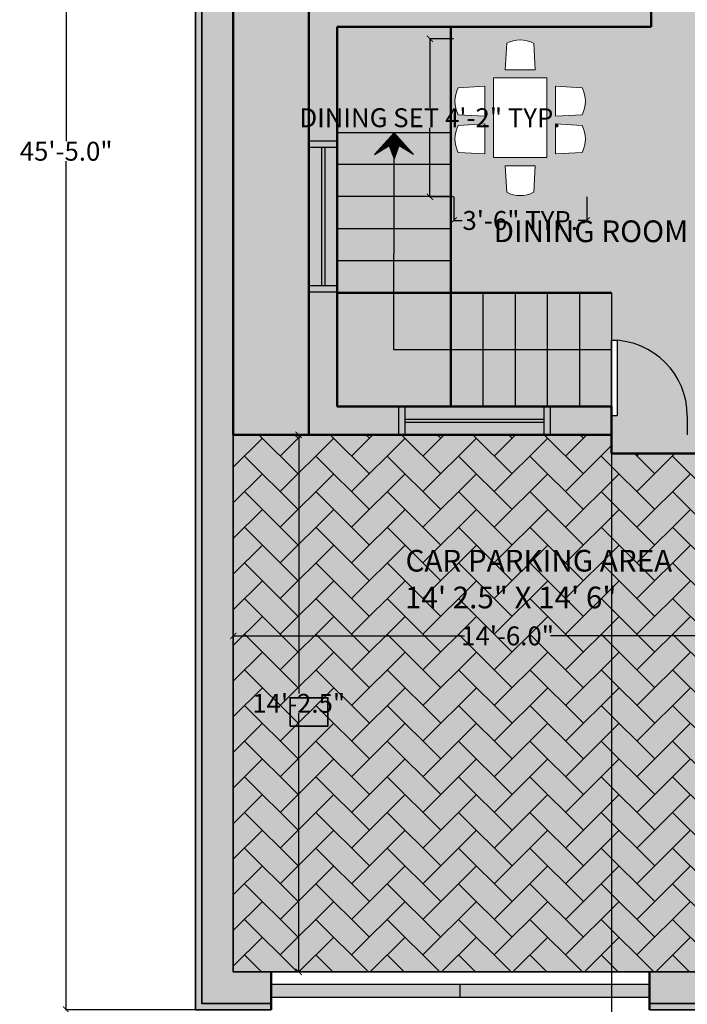
# Model space of a CAD drawing. Units: inches. Extents: x 528 to 2620, y -1066 to 798.
# Tile 2 of 41: x 528 to 740, y 211 to 523. Entities that reach past the tile are written whole.
import ezdxf

# ---------------------------------------------------------------- set-up
doc = ezdxf.new("R2010")
doc.units = ezdxf.units.IN
doc.header["$MEASUREMENT"] = 0
for name, color, linetype, lineweight in [('A-ANNO-DIMS', 2, 'Continuous', 18), ('A-AREA-IDEN', 7, 'Continuous', 18), ('A-COLS', 1, 'Continuous', 35), ('A-Door', 2, 'Continuous', 25), ('A-FLOR-PATT', 9, 'Continuous', 13), ('A-FLOR-STRS', 6, 'Continuous', 25), ('A-FURN', 30, 'Continuous', 18), ('A-GLAZ', 3, 'Continuous', 25), ('A-WALL', 7, 'Continuous', 50), ('A-WALL-PATT', 8, 'Continuous', 13), ('C-PROP', 5, 'Continuous', 35)]:
    doc.layers.add(name, color=color, linetype=linetype, lineweight=lineweight)
doc.styles.get("Standard").update_dxf_attribs({"font": 'arial.ttf'})
doc.dimstyles.get("Standard").update_dxf_attribs({"dimtxt": 6, "dimasz": 2, "dimexe": 0.18, "dimexo": 0.0625, "dimgap": 0.09, "dimtad": 0, "dimtih": 1, "dimtoh": 1, "dimdec": 1, "dimzin": 0, "dimdsep": 46, "dimlunit": 3, "dimtxsty": 'Standard', "dimblk": 'ARCHTICK', "dimcen": 0.09, "dimadec": 0, "dimazin": 0, "dimtfac": 1, "dimtdec": 1, "dimtofl": 0, "dimtmove": 0, "dimatfit": 3, "dimfxl": 1, "dimtolj": 1, "dimtzin": 0, "dimarcsym": 0})

# ---------------------------------------------------------------- blocks, each defined once
blk = doc.blocks.new('*U3')
for p, q in [((0, 0), (0, -6)), ((24, 0), (24, -6))]:
    blk.add_line(p, q)
blk.add_lwpolyline([(0, 0), (0, 24), (1.75, 24), (1.75, 0)], close=True)
blk.add_arc((0, 0), 24, 0, 90)
blk = doc.blocks.new('table-11')
at = {"color": 0, "linetype": 'ByBlock'}
for p, q in [((-1.122, 0.533), (-1.144, 0.134)), ((-0.716, 0.533), (-0.694, 0.134)), ((-0.554, 0.533), (-0.576, 0.134)), ((-0.148, 0.533), (-0.126, 0.134)), ((0, 0), (-1.2, 0)), ((-1.2, -0.8), (-1.2, 0)), ((-1.144, 0.134), (-0.694, 0.134)), ((-0.576, 0.134), (-0.126, 0.134)), ((0, -0.8), (0, 0)), ((-1.723, -0.197), (-1.324, -0.175)), ((-1.324, -0.625), (-1.324, -0.175)), ((0.523, -0.197), (0.124, -0.175)), ((0.124, -0.625), (0.124, -0.175)), ((-1.723, -0.603), (-1.324, -0.625)), ((0.523, -0.603), (0.124, -0.625)), ((0, -0.8), (-1.2, -0.8)), ((-1.144, -0.934), (-0.694, -0.934)), ((-1.122, -1.333), (-1.144, -0.934)), ((-0.716, -1.333), (-0.694, -0.934)), ((-0.576, -0.934), (-0.126, -0.934)), ((-0.554, -1.333), (-0.576, -0.934)), ((-0.148, -1.333), (-0.126, -0.934))]:
    blk.add_line(p, q, dxfattribs=at)
for centre, start, end in [((-0.919, 0.159), 61.4891, 118.5109), ((-0.351, 0.159), 61.4891, 118.5109), ((-1.349, -0.4), 151.4891, 208.5109), ((0.149, -0.4), 331.4891, 28.5109), ((-0.919, -0.959), 241.4891, 298.5109), ((-0.351, -0.959), 241.4891, 298.5109)]:
    blk.add_arc(centre, 0.425, start, end, dxfattribs=at)
blk = doc.blocks.new('_ArchTick')
at = {"color": 0, "linetype": 'ByBlock', "const_width": 0.15}
blk.add_lwpolyline([(-0.5, -0.5), (0.5, 0.5)], dxfattribs=at)
blk = doc.blocks.new('*D12')
at = {"layer": 'A-ANNO-DIMS', "color": 0, "lineweight": -2, "transparency": 16777216}
for p, q in [((584, 753.92), (542.88, 753.92)), ((543.06, 753.92), (543.06, 484.58)), ((543.06, 208.92), (543.06, 478.27)), ((584, 208.92), (542.88, 208.92))]:
    blk.add_line(p, q, dxfattribs=at)
at = {"layer": 'Defpoints', "color": 0, "transparency": 16777216}
for p in [(584.06, 753.92), (543.06, 208.92), (584.06, 208.92)]:
    blk.add_point(p, dxfattribs=at)
at = {"layer": 'A-ANNO-DIMS', "color": 0, "lineweight": -2, "transparency": 16777216, "xscale": 2, "yscale": 2, "zscale": 2}
for p, rotation in [((543.06, 753.92), 90), ((543.06, 208.92), 270)]:
    blk.add_blockref('_ArchTick', p, dxfattribs=dict(at, rotation=rotation))
at = {"layer": 'A-ANNO-DIMS', "color": 0, "transparency": 16777216, "insert": (543.06, 481.42), "char_height": 6, "attachment_point": 5}
blk.add_mtext('\\A1;45\'-5.0"', dxfattribs=at)
blk = doc.blocks.new('*D37')
at = {"layer": 'A-ANNO-DIMS', "color": 0, "lineweight": -2, "transparency": 16777216}
for p, q in [((596.06, 330.11), (596.06, 327.39)), ((770.06, 330.11), (770.06, 327.39)), ((596.06, 327.57), (669.45, 327.57)), ((770.06, 327.57), (696.67, 327.57))]:
    blk.add_line(p, q, dxfattribs=at)
at = {"layer": 'Defpoints', "color": 0, "transparency": 16777216}
for p in [(596.06, 330.17), (770.06, 330.17), (596.06, 327.57)]:
    blk.add_point(p, dxfattribs=at)
at = {"layer": 'A-ANNO-DIMS', "color": 0, "lineweight": -2, "transparency": 16777216, "xscale": 2, "yscale": 2, "zscale": 2, "rotation": 180}
blk.add_blockref('_ArchTick', (596.06, 327.57), dxfattribs=at)
at = {"layer": 'A-ANNO-DIMS', "color": 0, "lineweight": -2, "transparency": 16777216, "xscale": 2, "yscale": 2, "zscale": 2}
blk.add_blockref('_ArchTick', (770.06, 327.57), dxfattribs=at)
at = {"layer": 'A-ANNO-DIMS', "color": 0, "transparency": 16777216, "insert": (683.06, 327.57), "char_height": 6, "attachment_point": 5}
blk.add_mtext('\\A1;14\'-6.0"', dxfattribs=at)
blk = doc.blocks.new('*D38')
at = {"layer": 'A-ANNO-DIMS', "color": 0, "lineweight": -2, "transparency": 16777216}
for p, q in [((602.94, 391.42), (617, 391.42)), ((616.82, 391.42), (616.82, 309.33)), ((616.82, 220.92), (616.82, 303.02)), ((602.94, 220.92), (617, 220.92))]:
    blk.add_line(p, q, dxfattribs=at)
at = {"layer": 'Defpoints', "color": 0, "transparency": 16777216}
for p in [(602.87, 391.42), (602.87, 220.92), (616.82, 220.92)]:
    blk.add_point(p, dxfattribs=at)
at = {"layer": 'A-ANNO-DIMS', "color": 0, "lineweight": -2, "transparency": 16777216, "xscale": 2, "yscale": 2, "zscale": 2}
for p, rotation in [((616.82, 391.42), 90), ((616.82, 220.92), 270)]:
    blk.add_blockref('_ArchTick', p, dxfattribs=dict(at, rotation=rotation))
at = {"layer": 'A-ANNO-DIMS', "color": 0, "transparency": 16777216, "insert": (616.82, 306.17), "char_height": 6, "attachment_point": 5}
blk.add_mtext('\\A1;14\'-2.5"', dxfattribs=at)
blk = doc.blocks.new('WIN-1200')
for p, q in [((677.56, 718.92), (725.56, 718.92)), ((677.56, 709.92), (677.56, 718.92)), ((679.56, 709.92), (679.56, 718.92)), ((723.56, 718.92), (723.56, 709.92)), ((725.56, 718.92), (725.56, 709.92)), ((679.56, 714.92), (723.56, 714.92)), ((679.56, 713.92), (723.56, 713.92)), ((725.56, 709.92), (677.56, 709.92))]:
    blk.add_line(p, q)
blk = doc.blocks.new('*D48')
at = {"layer": 'A-ANNO-DIMS', "color": 0, "lineweight": -2, "transparency": 16777216}
for p, q in [((665.92, 517.14), (658.27, 517.14)), ((658.45, 517.14), (658.45, 495.24)), ((658.45, 466.96), (658.45, 488.86)), ((665.92, 466.96), (658.27, 466.96))]:
    blk.add_line(p, q, dxfattribs=at)
at = {"layer": 'Defpoints', "color": 0, "transparency": 16777216}
for p in [(658.45, 517.14), (665.98, 517.14), (665.98, 466.96)]:
    blk.add_point(p, dxfattribs=at)
at = {"layer": 'A-ANNO-DIMS', "color": 0, "lineweight": -2, "transparency": 16777216, "xscale": 2, "yscale": 2, "zscale": 2}
for p, rotation in [((658.45, 517.14), 90), ((658.45, 466.96), 270)]:
    blk.add_blockref('_ArchTick', p, dxfattribs=dict(at, rotation=rotation))
at = {"layer": 'A-ANNO-DIMS', "color": 0, "transparency": 16777216, "insert": (658.45, 492.05), "char_height": 6, "attachment_point": 5}
blk.add_mtext('\\A1;DINING SET 4\'-2" TYP.', dxfattribs=at)
blk = doc.blocks.new('*D49')
at = {"layer": 'A-ANNO-DIMS', "color": 0, "lineweight": -2, "transparency": 16777216}
for p, q in [((665.98, 466.9), (665.98, 459.26)), ((708.15, 466.9), (708.15, 459.26)), ((665.98, 459.44), (668.69, 459.44)), ((708.15, 459.44), (705.44, 459.44))]:
    blk.add_line(p, q, dxfattribs=at)
at = {"layer": 'Defpoints', "color": 0, "transparency": 16777216}
for p in [(665.98, 466.96), (708.15, 466.96), (665.98, 459.44)]:
    blk.add_point(p, dxfattribs=at)
at = {"layer": 'A-ANNO-DIMS', "color": 0, "lineweight": -2, "transparency": 16777216, "xscale": 2, "yscale": 2, "zscale": 2, "rotation": 180}
blk.add_blockref('_ArchTick', (665.98, 459.44), dxfattribs=at)
at = {"layer": 'A-ANNO-DIMS', "color": 0, "lineweight": -2, "transparency": 16777216, "xscale": 2, "yscale": 2, "zscale": 2}
blk.add_blockref('_ArchTick', (708.15, 459.44), dxfattribs=at)
at = {"layer": 'A-ANNO-DIMS', "color": 0, "transparency": 16777216, "insert": (687.06, 459.44), "char_height": 6, "attachment_point": 5}
blk.add_mtext('\\A1;3\'-6" TYP.', dxfattribs=at)
blk = doc.blocks.new('*D57')
at = {"layer": 'A-ANNO-DIMS', "color": 0, "lineweight": -2, "transparency": 16777216}
for p, q in [((716.06, 391.36), (716.06, 174.74)), ((764.06, 391.36), (764.06, 174.74)), ((716.06, 174.92), (731.87, 174.92)), ((764.06, 174.92), (748.24, 174.92))]:
    blk.add_line(p, q, dxfattribs=at)
at = {"layer": 'Defpoints', "color": 0, "transparency": 16777216}
for p in [(716.06, 391.42), (764.06, 391.42), (764.06, 174.92)]:
    blk.add_point(p, dxfattribs=at)
at = {"layer": 'A-ANNO-DIMS', "color": 0, "lineweight": -2, "transparency": 16777216, "xscale": 2, "yscale": 2, "zscale": 2, "rotation": 180}
blk.add_blockref('_ArchTick', (716.06, 174.92), dxfattribs=at)
at = {"layer": 'A-ANNO-DIMS', "color": 0, "lineweight": -2, "transparency": 16777216, "xscale": 2, "yscale": 2, "zscale": 2}
blk.add_blockref('_ArchTick', (764.06, 174.92), dxfattribs=at)
at = {"layer": 'A-ANNO-DIMS', "color": 0, "transparency": 16777216, "insert": (740.06, 174.92), "char_height": 6, "attachment_point": 5}
blk.add_mtext('\\A1;4\'-0"', dxfattribs=at)

msp = doc.modelspace()

# ---------------------------------------------------------------- hatches: boundary and pattern name
at = {"layer": 'A-COLS', "transparency": 33554687}
h = msp.add_hatch(color=256, dxfattribs=at)
h.dxf.hatch_style = 1
h.paths.add_polyline_path([(614.06, 307.96), (614.06, 298.96), (626.06, 298.96), (626.06, 307.96)])
at = {"layer": 'A-FLOR-PATT', "transparency": 33554607}
h = msp.add_hatch(dxfattribs=at)
h.set_pattern_fill('AR-HBONE', color=256, scale=2)
h.paths.add_polyline_path([(770.06, 391.42), (764.06, 391.42), (764.06, 385.42), (716.06, 385.42), (716.06, 391.42), (620.06, 391.42), (596.06, 391.42), (596.06, 220.92), (770.06, 220.92), (770.06, 268.92)])
at = {"layer": 'A-WALL-PATT', "transparency": 33554687}
h = msp.add_hatch(color=256, dxfattribs=at)
h.dxf.hatch_style = 1
h.paths.add_polyline_path([(944.06, 753.92), (584.06, 753.92), (584.06, 208.92), (608.06, 208.92), (608.06, 210.92), (586.06, 210.92), (586.06, 751.92), (942.06, 751.92), (942.06, 210.92), (728.06, 210.92), (728.06, 208.92), (944.06, 208.92)])
h = msp.add_hatch(color=256, dxfattribs=at)
h.dxf.hatch_style = 1
h.paths.add_polyline_path([(942.06, 751.92), (586.06, 751.92), (586.06, 210.92), (608.06, 210.92), (608.06, 220.92), (596.06, 220.92), (596.06, 741.92), (932.06, 741.92), (932.06, 220.92), (770.06, 220.92), (728.06, 220.92), (728.06, 210.92), (942.06, 210.92)])
at = {"layer": 'A-WALL-PATT', "transparency": 33554475}
h = msp.add_hatch(color=256, dxfattribs=at)
h.dxf.hatch_style = 1
h.paths.add_polyline_path([(620.06, 718.92), (908.06, 718.92), (908.06, 268.92), (770.06, 268.92), (770.06, 220.92), (932.06, 220.92), (932.06, 741.92), (596.06, 741.92), (596.06, 391.42), (620.06, 391.42)])
at = {"layer": 'A-WALL-PATT', "transparency": 33554687}
h = msp.add_hatch(color=256, dxfattribs=at)
h.dxf.hatch_style = 1
h.paths.add_polyline_path([(861.06, 273.92), (817.06, 273.92), (817.06, 272.92), (861.06, 272.92)])
h.paths.add_polyline_path([(817.06, 277.92), (815.06, 277.92), (815.06, 268.92), (817.06, 268.92)])
h.paths.add_polyline_path([(908.06, 397.92), (899.06, 397.92), (899.06, 395.92), (908.06, 395.92)])
h.paths.add_polyline_path([(908.06, 443.92), (899.06, 443.92), (899.06, 441.92), (908.06, 441.92)])
h.paths.add_polyline_path([(904.06, 441.92), (903.06, 441.92), (903.06, 397.92), (904.06, 397.92)])
h.paths.add_polyline_path([(625.06, 561.42), (624.06, 561.42), (624.06, 537.42), (625.06, 537.42)])
h.paths.add_polyline_path([(648.75, 334.44), (720.04, 334.44), (720.04, 345), (648.75, 345)], flags=9)
h.paths.add_polyline_path([(819.73, 323.15), (880.33, 323.15), (880.33, 333.71), (819.73, 333.71)], flags=9)
h.paths.add_polyline_path([(779.9, 680.61), (821.76, 680.61), (821.76, 691.17), (779.9, 691.17)], flags=9)
h.paths.add_polyline_path([(779.88, 692.36), (817.14, 692.36), (817.14, 703.06), (779.88, 703.06)], flags=9)
h.paths.add_polyline_path([(799.99, 453.88), (860.59, 453.88), (860.59, 464.44), (799.99, 464.44)], flags=9)
h.paths.add_polyline_path([(650.87, 539.4), (708.78, 539.4), (708.78, 549.95), (650.87, 549.95)], flags=9)
h.paths.add_polyline_path([(788.5, 612.01), (849.1, 612.01), (849.1, 622.56), (788.5, 622.56)], flags=9)
h.paths.add_polyline_path([(639.54, 648.31), (700.13, 648.31), (700.13, 658.87), (639.54, 658.87)], flags=9)
h.paths.add_polyline_path([(648.91, 346.09), (747.71, 346.09), (747.71, 356.78), (648.91, 356.78)], flags=9)
h.paths.add_polyline_path([(676.86, 450.66), (746.74, 450.66), (746.74, 461.36), (676.86, 461.36)], flags=9)
h.paths.add_polyline_path([(819.71, 334.95), (865.53, 334.95), (865.53, 345.64), (819.71, 345.64)], flags=9)
h.paths.add_polyline_path([(806.3, 467.75), (874.05, 467.75), (874.05, 478.44), (806.3, 478.44)], flags=9)
h.paths.add_polyline_path([(653.23, 552.28), (690.5, 552.28), (690.5, 562.98), (653.23, 562.98)], flags=9)
h.paths.add_polyline_path([(789.9, 623.41), (843.21, 623.41), (843.21, 634.1), (789.9, 634.1)], flags=9)
h.paths.add_polyline_path([(639.77, 662.1), (693.08, 662.1), (693.08, 672.8), (639.77, 672.8)], flags=9)
h.paths.add_polyline_path([(801.59, 242.91), (846.33, 242.91), (846.33, 253.6), (801.59, 253.6)], flags=9)
h.paths.add_polyline_path([(925.36, 593.98), (925.36, 674.06), (914.67, 674.06), (914.67, 593.98)], flags=9)
h.paths.add_polyline_path([(612.56, 593.98), (612.56, 674.06), (601.87, 674.06), (601.87, 593.98)], flags=9)
h.paths.add_polyline_path([(723.31, 726.56), (803.39, 726.56), (803.39, 737.25), (723.31, 737.25)], flags=9)
at = {"layer": 'A-WALL-PATT', "transparency": 33554521}
h = msp.add_hatch(color=256, dxfattribs=at)
h.dxf.hatch_style = 1
h.paths.add_polyline_path([(629.06, 709.92), (677.56, 709.92), (677.56, 718.92), (620.06, 718.92), (620.06, 667.92), (629.06, 667.92)])
h.paths.add_polyline_path([(790.56, 718.92), (725.56, 718.92), (725.56, 709.92), (774.06, 709.92), (774.06, 577.92), (768.48, 577.92), (768.56, 573.42), (774.06, 573.42), (774.06, 567.42), (778.56, 567.42), (778.56, 669.42), (831.06, 669.42), (831.06, 675.92), (826.56, 675.92), (826.56, 673.92), (778.56, 673.92), (778.56, 709.92), (790.56, 709.92)])
h.paths.add_polyline_path([(908.06, 718.92), (879.06, 718.92), (879.06, 709.92), (899.06, 709.92), (899.06, 641.67), (908.06, 641.67)])
h.paths.add_polyline_path([(629.06, 619.92), (620.06, 619.92), (620.06, 561.42), (629.06, 561.42), (629.06, 573.42), (724.06, 573.42), (724.06, 569.42), (728.56, 569.42), (728.56, 577.92), (629.06, 577.92)])
h.paths.add_polyline_path([(779.06, 391.42), (779.06, 400.42), (770.06, 400.42), (764.06, 400.42), (764.06, 397.42), (764.06, 391.42), (770.06, 391.42), (770.06, 268.92), (815.06, 268.92), (815.06, 277.92), (779.06, 277.92), (779.06, 359.77)])
h.paths.add_polyline_path([(908.06, 395.92), (899.06, 395.92), (851.06, 395.92), (851.06, 391.42), (899.06, 391.42), (899.06, 277.92), (863.06, 277.92), (863.06, 268.92), (908.06, 268.92)])
h.paths.add_polyline_path([(908.06, 593.67), (899.06, 593.67), (899.06, 525.42), (778.56, 525.42), (778.56, 527.17), (774.06, 527.17), (774.06, 520.92), (899.06, 520.92), (899.06, 443.92), (908.06, 443.92)])
h.paths.add_polyline_path([(629.06, 520.92), (728.56, 520.92), (728.56, 545.42), (724.06, 545.42), (724.06, 525.42), (629.06, 525.42), (629.06, 537.42), (620.06, 537.42), (620.06, 484.67), (629.06, 484.67)])
h.paths.add_polyline_path([(629.06, 436.67), (620.06, 436.67), (620.06, 391.42), (648.56, 391.42), (648.56, 400.42), (629.06, 400.42)])
h.paths.add_polyline_path([(716.06, 397.42), (716.06, 400.42), (696.56, 400.42), (696.56, 391.42), (716.06, 391.42)])
at = {"layer": 'A-WALL-PATT', "transparency": 33554681}
h = msp.add_hatch(color=256, dxfattribs=at)
h.dxf.hatch_style = 1
h.paths.add_polyline_path([(629.06, 665.92), (625.06, 665.92), (625.06, 621.92), (629.06, 621.92)])
h.paths.add_polyline_path([(624.06, 665.92), (620.06, 665.92), (620.06, 621.92), (624.06, 621.92)])
h.paths.add_polyline_path([(723.56, 713.92), (679.56, 713.92), (679.56, 709.92), (723.56, 709.92)])
h.paths.add_polyline_path([(723.56, 718.92), (679.56, 718.92), (679.56, 714.92), (723.56, 714.92)])
h.paths.add_polyline_path([(814.56, 713.92), (790.56, 713.92), (790.56, 709.92), (814.56, 709.92)])
h.paths.add_polyline_path([(814.56, 718.92), (790.56, 718.92), (790.56, 714.92), (814.56, 714.92)])
h.paths.add_polyline_path([(877.06, 713.92), (833.06, 713.92), (833.06, 709.92), (877.06, 709.92)])
h.paths.add_polyline_path([(877.06, 718.92), (833.06, 718.92), (833.06, 714.92), (877.06, 714.92)])
h.paths.add_polyline_path([(908.06, 639.67), (904.06, 639.67), (904.06, 595.67), (908.06, 595.67)])
h.paths.add_polyline_path([(903.06, 639.67), (899.06, 639.67), (899.06, 595.67), (903.06, 595.67)])
h.paths.add_polyline_path([(908.06, 441.92), (904.06, 441.92), (904.06, 397.92), (908.06, 397.92)])
h.paths.add_polyline_path([(903.06, 441.92), (899.06, 441.92), (899.06, 397.92), (903.06, 397.92)])
h.paths.add_polyline_path([(861.06, 272.92), (817.06, 272.92), (817.06, 268.92), (861.06, 268.92)])
h.paths.add_polyline_path([(861.06, 277.92), (817.06, 277.92), (817.06, 273.92), (861.06, 273.92)])
h.paths.add_polyline_path([(694.56, 395.42), (650.56, 395.42), (650.56, 391.42), (694.56, 391.42)])
h.paths.add_polyline_path([(694.56, 400.42), (650.56, 400.42), (650.56, 396.42), (694.56, 396.42)])
h.paths.add_polyline_path([(629.06, 482.67), (625.06, 482.67), (625.06, 438.67), (629.06, 438.67)])
h.paths.add_polyline_path([(624.06, 482.67), (620.06, 482.67), (620.06, 438.67), (624.06, 438.67)])
h.paths.add_polyline_path([(629.06, 561.42), (625.06, 561.42), (625.06, 537.42), (629.06, 537.42)])
h.paths.add_polyline_path([(624.06, 561.42), (620.06, 561.42), (620.06, 537.42), (624.06, 537.42)])
h = msp.add_hatch(color=256, dxfattribs=at)
h.dxf.hatch_style = 1
h.paths.add_polyline_path([(625.06, 665.92), (624.06, 665.92), (624.06, 621.92), (625.06, 621.92)])
h.paths.add_polyline_path([(629.06, 667.92), (620.06, 667.92), (620.06, 665.92), (629.06, 665.92)])
h.paths.add_polyline_path([(629.06, 621.92), (620.06, 621.92), (620.06, 619.92), (629.06, 619.92)])
h.paths.add_polyline_path([(723.56, 714.92), (679.56, 714.92), (679.56, 713.92), (723.56, 713.92)])
h.paths.add_polyline_path([(725.56, 718.92), (723.56, 718.92), (723.56, 709.92), (725.56, 709.92)])
h.paths.add_polyline_path([(679.56, 718.92), (677.56, 718.92), (677.56, 709.92), (679.56, 709.92)])
h.paths.add_polyline_path([(814.56, 714.92), (790.56, 714.92), (790.56, 713.92), (814.56, 713.92)])
h.paths.add_polyline_path([(877.06, 714.92), (833.06, 714.92), (833.06, 713.92), (877.06, 713.92)])
h.paths.add_polyline_path([(879.06, 718.92), (877.06, 718.92), (877.06, 709.92), (879.06, 709.92)])
h.paths.add_polyline_path([(833.06, 718.92), (831.06, 718.92), (831.06, 709.92), (833.06, 709.92)])
h.paths.add_polyline_path([(650.56, 400.42), (648.56, 400.42), (648.56, 391.42), (650.56, 391.42)])
h.paths.add_polyline_path([(694.56, 396.42), (650.56, 396.42), (650.56, 395.42), (694.56, 395.42)])
h.paths.add_polyline_path([(696.56, 400.42), (694.56, 400.42), (694.56, 391.42), (696.56, 391.42)])
h.paths.add_polyline_path([(629.06, 438.67), (620.06, 438.67), (620.06, 436.67), (629.06, 436.67)])
h.paths.add_polyline_path([(629.06, 484.67), (620.06, 484.67), (620.06, 482.67), (629.06, 482.67)])
h.paths.add_polyline_path([(625.06, 482.67), (624.06, 482.67), (624.06, 438.67), (625.06, 438.67)])
at = {"layer": 'A-WALL-PATT', "transparency": 33554590}
h = msp.add_hatch(color=256, dxfattribs=at)
h.dxf.hatch_style = 1
h.paths.add_polyline_path([(774.06, 709.92), (629.06, 709.92), (629.06, 577.92), (728.56, 577.92), (728.56, 579.42), (728.56, 619.42), (730.31, 619.42), (730.31, 619.38, -0.401453), (768.56, 579.42), (768.56, 577.92), (774.06, 577.92)])
h.paths.add_polyline_path([(723.9, 686.06), (723.97, 686.06), (723.83, 686.13)], flags=0)
h.paths.add_polyline_path([(722.79, 642.7), (722.89, 642.76), (722.89, 684.99), (722.65, 685.24), (722.65, 685.82), (723.08, 686.26), (723.53, 686.26), (723.97, 686.06), (724.74, 686.13), (770.7, 686.13), (770.78, 686.14), (771.13, 686.27), (771.69, 686.09), (771.94, 685.48), (771.67, 684.9), (771.58, 684.87), (771.58, 642.78), (771.88, 642.51), (771.88, 641.92), (771.51, 641.46), (770.85, 641.46), (770.4, 641.83), (770.4, 641.55), (724.74, 641.55), (723.99, 641.7), (723.44, 641.41), (722.88, 641.59), (722.6, 642.14)], flags=16)
h.paths.add_polyline_path([(723.99, 641.7), (723.99, 641.71), (723.99, 641.7)], flags=0)
h.paths.add_polyline_path([(722.89, 642.73), (722.89, 684.99), (722.65, 685.24), (722.65, 685.82), (723.08, 686.26), (723.29, 686.26), (722.99, 686.17), (722.79, 685.97), (722.65, 685.68), (722.65, 685.43), (722.75, 685.14), (722.94, 684.94), (723.24, 684.81), (723.48, 684.81), (723.78, 684.9), (723.98, 685.1), (724.17, 685.49), (724.12, 685.64), (724.12, 685.25), (723.63, 684.75), (723.63, 642.96), (724.12, 642.51), (724.12, 641.89), (723.66, 641.46), (723.08, 641.46), (722.65, 641.9), (722.65, 642.48)], flags=0)
h.paths.add_polyline_path([(722.65, 642.29), (722.65, 642.04), (722.79, 641.75), (723.08, 641.46), (723.29, 641.46), (722.88, 641.59), (722.6, 642.14)], flags=0)
h.paths.add_polyline_path([(770.75, 686.13), (770.58, 686.13), (770.55, 686.06)], flags=0)
h.paths.add_polyline_path([(743.3, 645.29), (753.23, 659.4), (748.69, 663.75), (753.23, 668.54), (743.3, 682.46), (743.79, 682.59), (744.14, 682.68), (744.53, 682.93), (744.63, 683.08), (745.02, 683.33), (744.53, 684.07), (744.78, 684.16), (744.87, 684.31), (745.51, 684.4), (746.08, 684.65), (746.47, 684.65), (746.82, 684.81), (747.46, 685.03), (747.71, 685.14), (748.2, 685.28), (748.39, 685.52), (748.86, 685.52), (749.99, 686.13), (753.49, 676.03), (757.38, 680.15), (757.79, 679.76), (758.04, 680.65), (758.29, 681.23), (758.29, 682.05), (758.02, 682.59), (757.87, 683.17), (757.82, 683.78), (758.39, 684.07), (758.98, 684.2), (759.62, 684.16), (760.21, 683.96), (760.75, 683.67), (761.86, 683.67), (762.4, 683.96), (762.99, 684.11), (763.63, 684.11), (764.2, 683.96), (764.74, 683.67), (766.12, 683.67), (766.66, 683.96), (767.25, 684.16), (767.87, 684.2), (768.46, 684.07), (769.05, 683.78), (769, 683.17), (768.85, 682.59), (768.55, 682.05), (768.55, 681.23), (768.8, 680.65), (769.09, 679.75), (768.95, 678.83), (768.8, 678.23), (768.55, 677.65), (768.55, 676.82), (768.8, 676.24), (769.09, 675.34), (768.95, 674.42), (768.8, 673.82), (768.55, 673.28), (768.55, 672.41), (768.8, 671.87), (769, 671.29), (769.05, 670.64), (768.95, 670.02), (768.8, 669.41), (768.55, 668.87), (768.55, 668), (768.97, 667.24), (769.05, 666.28), (769.05, 665.56), (768.46, 665.32), (767.87, 665.16), (767.25, 665.16), (766.66, 665.36), (766.12, 665.7), (764.74, 665.7), (763.94, 665.2), (762.99, 665.2), (762.4, 665.36), (761.86, 665.7), (761, 665.7), (762.7, 664.09), (760.74, 662.03), (761.86, 662.03), (762.4, 662.32), (763.34, 662.55), (764.25, 662.32), (764.79, 662.03), (766.12, 662.03), (766.66, 662.32), (767.25, 662.52), (767.87, 662.56), (768.51, 662.43), (769.05, 662.12), (769.05, 661.4), (769.05, 660.8), (768.85, 660.21), (768.55, 659.68), (768.55, 658.85), (768.85, 658.27), (769, 657.66), (769.07, 656.75), (768.85, 655.85), (768.55, 655.27), (768.55, 654.44), (768.85, 653.86), (769.07, 652.96), (769, 652.05), (768.85, 651.44), (768.55, 650.91), (768.55, 650.03), (768.85, 649.5), (769, 648.91), (769.05, 648.26), (769, 647.64), (768.85, 647.03), (768.55, 646.5), (768.55, 645.62), (768.85, 645.09), (769.05, 644.55), (769.05, 643.9), (768.51, 643.65), (767.87, 643.52), (767.25, 643.52), (766.66, 643.72), (766.12, 644.06), (764.79, 644.06), (764.25, 643.72), (763.34, 643.49), (762.4, 643.72), (761.86, 644.06), (760.8, 644.06), (760.26, 643.72), (759.67, 643.52), (759.03, 643.52), (758.39, 643.65), (757.87, 643.9), (757.87, 644.55), (758.04, 645.09), (758.34, 645.62), (758.34, 646.5), (758.04, 647.03), (757.92, 647.64), (757.87, 648.06), (757.38, 647.59), (753.42, 651.77), (749.99, 641.62), (749.5, 641.71), (749.35, 641.95), (748.54, 642.45), (747.31, 642.94), (746.65, 642.94), (746.33, 643.18), (745.51, 643.57), (744.53, 643.65), (745.01, 644.4), (744.63, 644.64), (744.14, 644.89), (743.79, 645.13)], flags=0)
h.paths.add_polyline_path([(755.66, 654.93), (756.54, 654.69), (757.53, 654.33), (756.64, 654.58)], flags=0)
h.paths.add_polyline_path([(758.34, 649.2), (758.34, 648.71), (758.59, 644.3), (758.59, 648.8)], flags=0)
h.paths.add_polyline_path([(758.34, 649.29), (758.09, 649.7), (758.36, 649.17)], flags=0)
h.paths.add_polyline_path([(755.66, 672.79), (756.49, 673.04), (757.36, 673.35), (757.35, 673.36), (756.64, 673.15)], flags=0)
h.paths.add_polyline_path([(760.26, 639.64), (771.41, 639.64), (771.41, 624.04), (760.26, 624.04)], flags=16)
h.paths.add_polyline_path([(761.38, 638.53), (770.29, 638.53), (770.29, 625.15), (761.38, 625.15)], flags=0)
edge = h.paths.add_edge_path(flags=0)
edge.add_ellipse((765.84, 631.84), major_axis=(-2.24, 2.24), ratio=1, start_angle=-45, end_angle=45, ccw=False)
edge.add_ellipse((765.84, 631.84), major_axis=(-2.24, 2.24), ratio=1, start_angle=-135, end_angle=-45, ccw=False)
edge.add_ellipse((765.84, 631.84), major_axis=(-2.24, 2.24), ratio=1, start_angle=135, end_angle=-135, ccw=False)
edge.add_ellipse((765.84, 631.84), major_axis=(-2.24, 2.24), ratio=1, start_angle=45, end_angle=135, ccw=False)
h.paths.add_polyline_path([(758.59, 683.42), (758.59, 678.92), (758.37, 678.58), (758.34, 678.43), (758.09, 678.05), (758.34, 678.52), (758.34, 679.01)], flags=0)
h.paths.add_polyline_path([(760.26, 688.04), (760.26, 703.64), (771.41, 703.64), (771.41, 688.04)], flags=16)
h.paths.add_polyline_path([(770.4, 685.39), (770.4, 685.85), (770.85, 686.22), (771.51, 686.22), (771.88, 685.76), (771.88, 685.17), (771.58, 684.9), (771.58, 642.78), (771.88, 642.51), (771.88, 641.92), (771.51, 641.46), (770.85, 641.46), (770.4, 641.83), (770.4, 642.29)], flags=0)
h.paths.add_polyline_path([(770.53, 642.68), (771.05, 643.01), (771.67, 642.77), (771.94, 642.2), (771.69, 641.59), (771.13, 641.41), (770.55, 641.62), (770.35, 642.13)], flags=16)
h.paths.add_polyline_path([(761.38, 689.15), (761.38, 702.53), (770.29, 702.53), (770.29, 689.15)], flags=0)
edge = h.paths.add_edge_path(flags=0)
edge.add_ellipse((765.84, 695.84), major_axis=(2.24, 2.24), ratio=1, start_angle=405, end_angle=495, ccw=False)
edge.add_ellipse((765.84, 695.84), major_axis=(2.24, 2.24), ratio=1, start_angle=675, end_angle=765, ccw=False)
edge.add_ellipse((765.84, 695.84), major_axis=(2.24, 2.24), ratio=1, start_angle=585, end_angle=675, ccw=False)
edge.add_ellipse((765.84, 695.84), major_axis=(2.24, 2.24), ratio=1, start_angle=495, end_angle=585, ccw=False)
h.paths.add_polyline_path([(770.7, 684.9), (770.94, 684.74), (771.41, 684.74), (771.73, 685.03), (771.88, 685.34), (771.88, 685.64), (771.69, 686.09), (771.58, 686.13), (771.88, 685.76), (771.88, 685.17), (771.41, 684.74), (770.85, 684.74)], flags=0)
h.paths.add_polyline_path([(899.06, 709.92), (831.06, 709.92), (831.06, 699.92), (829.81, 699.92), (829.81, 675.92), (831.06, 675.92), (831.06, 669.42), (778.56, 669.42), (778.56, 567.17), (780.06, 567.17), (820.06, 567.17), (820.06, 565.42), (820.02, 565.42, -0.401453), (780.06, 527.17), (778.56, 527.17), (778.56, 525.42), (899.06, 525.42)])
h.paths.add_polyline_path([(849.2, 636.01), (849.27, 636.02), (849.13, 636.08)], flags=0)
h.paths.add_polyline_path([(848.19, 634.95), (847.95, 635.2), (847.95, 635.78), (848.38, 636.22), (848.83, 636.22), (849.27, 636.02), (850.04, 636.08), (896, 636.08), (896.08, 636.1), (896.43, 636.22), (896.99, 636.05), (897.24, 635.43), (896.97, 634.86), (896.88, 634.83), (896.88, 592.74), (897.18, 592.47), (897.18, 591.88), (896.81, 591.42), (896.15, 591.42), (895.7, 591.79), (895.7, 591.51), (850.04, 591.51), (849.29, 591.66), (848.74, 591.37), (848.18, 591.54), (847.9, 592.1), (848.09, 592.65), (848.19, 592.71)], flags=16)
h.paths.add_polyline_path([(849.29, 591.66), (849.29, 591.66), (849.29, 591.66)], flags=16)
h.paths.add_polyline_path([(848.19, 634.95), (847.95, 635.2), (847.95, 635.78), (848.38, 636.22), (848.59, 636.22), (848.29, 636.13), (848.09, 635.93), (847.95, 635.64), (847.95, 635.39), (848.05, 635.1), (848.24, 634.9), (848.54, 634.76), (848.78, 634.76), (849.08, 634.85), (849.28, 635.05), (849.47, 635.44), (849.42, 635.59), (849.42, 635.21), (848.93, 634.7), (848.93, 592.92), (849.42, 592.47), (849.42, 591.84), (848.96, 591.42), (848.38, 591.42), (847.95, 591.86), (847.95, 592.44), (848.19, 592.69)], flags=0)
h.paths.add_polyline_path([(847.95, 592.25), (847.95, 592), (848.09, 591.71), (848.38, 591.42), (848.59, 591.42), (848.18, 591.54), (847.9, 592.1)], flags=16)
h.paths.add_polyline_path([(896.05, 636.08), (895.88, 636.08), (895.85, 636.01)], flags=0)
h.paths.add_polyline_path([(868.6, 632.41), (869.09, 632.55), (869.44, 632.64), (869.83, 632.88), (869.93, 633.04), (870.32, 633.28), (869.83, 634.02), (870.08, 634.11), (870.17, 634.27), (870.81, 634.36), (871.38, 634.61), (871.77, 634.61), (872.12, 634.76), (872.76, 634.99), (873.01, 635.1), (873.5, 635.23), (873.69, 635.48), (874.16, 635.48), (875.29, 636.08), (878.79, 625.99), (882.68, 630.11), (883.09, 629.71), (883.34, 630.6), (883.59, 631.18), (883.59, 632.01), (883.32, 632.55), (883.17, 633.13), (883.12, 633.73), (883.69, 634.02), (884.28, 634.16), (884.92, 634.11), (885.51, 633.91), (886.05, 633.62), (887.16, 633.62), (887.7, 633.91), (888.29, 634.07), (888.93, 634.07), (889.5, 633.91), (890.04, 633.62), (891.42, 633.62), (891.96, 633.91), (892.55, 634.11), (893.17, 634.16), (893.76, 634.02), (894.35, 633.73), (894.3, 633.13), (894.15, 632.55), (893.85, 632.01), (893.85, 631.18), (894.1, 630.6), (894.39, 629.71), (894.25, 628.79), (894.1, 628.18), (893.85, 627.6), (893.85, 626.77), (894.1, 626.19), (894.39, 625.3), (894.25, 624.38), (894.1, 623.78), (893.85, 623.24), (893.85, 622.37), (894.1, 621.83), (894.3, 621.25), (894.35, 620.6), (894.25, 619.97), (894.1, 619.37), (893.85, 618.83), (893.85, 617.96), (894.27, 617.2), (894.35, 616.23), (894.35, 615.52), (893.76, 615.27), (893.17, 615.12), (892.55, 615.12), (891.96, 615.32), (891.42, 615.65), (890.04, 615.65), (889.25, 615.16), (888.29, 615.16), (887.7, 615.32), (887.16, 615.65), (886.31, 615.65), (888, 614.04), (886.04, 611.98), (887.16, 611.98), (887.7, 612.27), (888.64, 612.5), (889.55, 612.27), (890.09, 611.98), (891.42, 611.98), (891.96, 612.27), (892.55, 612.48), (893.17, 612.52), (893.81, 612.39), (894.35, 612.07), (894.35, 611.36), (894.35, 610.75), (894.15, 610.17), (893.85, 609.63), (893.85, 608.81), (894.15, 608.22), (894.3, 607.62), (894.37, 606.7), (894.15, 605.81), (893.85, 605.22), (893.85, 604.4), (894.15, 603.81), (894.37, 602.92), (894.3, 602), (894.15, 601.4), (893.85, 600.86), (893.85, 599.99), (894.15, 599.45), (894.3, 598.87), (894.35, 598.22), (894.3, 597.59), (894.15, 596.99), (893.85, 596.45), (893.85, 595.58), (894.15, 595.04), (894.35, 594.51), (894.35, 593.86), (893.81, 593.61), (893.17, 593.48), (892.55, 593.48), (891.96, 593.68), (891.42, 594.01), (890.09, 594.01), (889.55, 593.68), (888.64, 593.45), (887.7, 593.68), (887.16, 594.01), (886.1, 594.01), (885.56, 593.68), (884.97, 593.48), (884.33, 593.48), (883.69, 593.61), (883.17, 593.86), (883.17, 594.51), (883.34, 595.04), (883.64, 595.58), (883.64, 596.45), (883.34, 596.99), (883.22, 597.59), (883.17, 598.01), (882.68, 597.55), (878.72, 601.73), (875.29, 591.57), (874.8, 591.66), (874.65, 591.91), (873.84, 592.4), (872.61, 592.89), (871.95, 592.89), (871.63, 593.14), (870.81, 593.52), (869.83, 593.61), (870.31, 594.36), (869.93, 594.6), (869.44, 594.84), (869.09, 595.09), (868.6, 595.24), (878.53, 609.35), (873.99, 613.71), (878.53, 618.49)], flags=0)
h.paths.add_polyline_path([(880.96, 622.75), (881.79, 622.99), (882.66, 623.31), (882.65, 623.31), (881.94, 623.1)], flags=0)
h.paths.add_polyline_path([(880.96, 604.89), (881.84, 604.64), (882.83, 604.28), (881.94, 604.53)], flags=16)
h.paths.add_polyline_path([(883.39, 628.01), (883.64, 628.48), (883.64, 628.97), (883.89, 633.38), (883.89, 628.88), (883.67, 628.53), (883.64, 628.39)], flags=0)
h.paths.add_polyline_path([(883.64, 599.16), (883.64, 598.67), (883.89, 594.26), (883.89, 598.76)], flags=16)
h.paths.add_polyline_path([(883.64, 599.25), (883.39, 599.65), (883.66, 599.12)], flags=16)
h.paths.add_polyline_path([(885.56, 637.99), (885.56, 653.6), (896.71, 653.6), (896.71, 637.99)], flags=16)
h.paths.add_polyline_path([(885.56, 589.6), (896.71, 589.6), (896.71, 573.99), (885.56, 573.99)], flags=16)
h.paths.add_polyline_path([(886.68, 639.11), (886.68, 652.48), (895.59, 652.48), (895.59, 639.11)], flags=0)
h.paths.add_polyline_path([(886.68, 588.48), (895.59, 588.48), (895.59, 575.11), (886.68, 575.11)], flags=0)
edge = h.paths.add_edge_path(flags=0)
edge.add_ellipse((891.14, 645.79), major_axis=(2.24, 2.24), ratio=1, start_angle=405, end_angle=495, ccw=False)
edge.add_ellipse((891.14, 645.79), major_axis=(2.24, 2.24), ratio=1, start_angle=675, end_angle=765, ccw=False)
edge.add_ellipse((891.14, 645.79), major_axis=(2.24, 2.24), ratio=1, start_angle=585, end_angle=675, ccw=False)
edge.add_ellipse((891.14, 645.79), major_axis=(2.24, 2.24), ratio=1, start_angle=495, end_angle=585, ccw=False)
edge = h.paths.add_edge_path(flags=0)
edge.add_ellipse((891.14, 581.8), major_axis=(-2.24, 2.24), ratio=1, start_angle=-45, end_angle=45, ccw=False)
edge.add_ellipse((891.14, 581.8), major_axis=(-2.24, 2.24), ratio=1, start_angle=-135, end_angle=-45, ccw=False)
edge.add_ellipse((891.14, 581.8), major_axis=(-2.24, 2.24), ratio=1, start_angle=135, end_angle=-135, ccw=False)
edge.add_ellipse((891.14, 581.8), major_axis=(-2.24, 2.24), ratio=1, start_angle=45, end_angle=135, ccw=False)
h.paths.add_polyline_path([(895.7, 635.35), (895.7, 635.8), (896.15, 636.17), (896.81, 636.17), (897.18, 635.71), (897.18, 635.12), (896.88, 634.85), (896.88, 592.74), (897.18, 592.47), (897.18, 591.88), (896.81, 591.42), (896.15, 591.42), (895.7, 591.79), (895.7, 592.25)], flags=0)
h.paths.add_polyline_path([(896, 634.85), (896.24, 634.7), (896.71, 634.7), (897.03, 634.99), (897.18, 635.3), (897.18, 635.59), (896.99, 636.05), (896.88, 636.08), (897.18, 635.71), (897.18, 635.12), (896.71, 634.7), (896.15, 634.7)], flags=0)
h.paths.add_polyline_path([(895.83, 592.63), (896.35, 592.96), (896.97, 592.73), (897.24, 592.16), (896.99, 591.54), (896.43, 591.37), (895.85, 591.58), (895.65, 592.09)], flags=16)
h.paths.add_polyline_path([(725.25, 569.42), (724.06, 569.42), (724.06, 573.42), (629.06, 573.42), (629.06, 525.42), (724.06, 525.42), (724.06, 545.42), (725.25, 545.42)])
h.paths.add_polyline_path([(820.02, 565.42), (780.06, 565.42), (780.06, 567.17), (774.06, 567.17), (774.06, 567.42), (774.06, 573.42), (768.56, 573.42), (768.48, 577.92), (768.56, 577.92), (768.56, 579.42, 0.401453), (730.31, 619.38), (730.31, 579.42), (728.56, 579.42), (728.56, 573.42), (728.56, 569.42), (727.25, 569.42), (727.25, 545.42), (728.56, 545.42), (728.56, 520.92), (665.06, 520.92), (665.06, 436.42), (716.06, 436.42), (716.06, 421.42), (717.81, 421.42), (717.81, 421.36, -0.392996), (740.06, 397.42, -0.392996), (762.31, 421.36), (762.31, 421.42), (764.06, 421.42), (764.06, 400.42), (770.06, 400.42), (779.06, 400.42), (779.06, 391.42), (779.06, 359.77), (795.43, 359.77), (795.43, 294.3), (893.67, 294.3), (893.67, 277.92), (899.06, 277.92), (899.06, 391.42), (851.06, 391.42), (851.06, 395.92), (899.06, 395.92), (899.06, 443.92), (899.06, 520.92), (774.06, 520.92), (774.06, 527.17), (778.56, 527.17), (780.06, 527.17, 0.401453)])
h.paths.add_polyline_path([(774.06, 519.66), (842.12, 519.66), (842.12, 505.07), (788.64, 505.07), (788.64, 474.08), (788.64, 470.43, -0.883215), (779.53, 456.66), (774.97, 456.66, -0.414214), (774.06, 457.57)], flags=16)
h.paths.add_polyline_path([(775.88, 517.83), (840.3, 517.83), (840.3, 514.19), (788.64, 514.19), (788.64, 484.41), (779.53, 484.41), (779.53, 474.08), (775.88, 474.08)], flags=0)
h.paths.add_polyline_path([(706.7, 501.56, -0.254069), (706.7, 493.02), (698.31, 492.55), (698.31, 502.03)], flags=16)
h.paths.add_polyline_path([(691.33, 515.69), (691.8, 507.3), (682.32, 507.3), (682.79, 515.69, -0.254069)], flags=16)
h.paths.add_polyline_path([(695.49, 504.68), (695.49, 479.42), (678.64, 479.42), (678.64, 504.68)], flags=16)
h.paths.add_polyline_path([(706.7, 489.6, -0.254069), (706.7, 481.06), (698.31, 480.59), (698.31, 490.07)], flags=16)
h.paths.add_polyline_path([(675.81, 502.03), (675.81, 492.55), (667.42, 493.02, -0.254069), (667.42, 501.56)], flags=16)
h.paths.add_polyline_path([(691.8, 476.8), (691.33, 468.41, -0.254069), (682.79, 468.41), (682.32, 476.8)], flags=16)
h.paths.add_polyline_path([(675.81, 490.07), (675.81, 480.59), (667.42, 481.06, -0.254069), (667.42, 489.6)], flags=16)
h.paths.add_polyline_path([(764.06, 397.42), (762.31, 397.42), (762.31, 421.36, 0.392996), (740.06, 397.42, 0.392996), (717.81, 421.36), (717.81, 397.42), (716.06, 397.42), (716.06, 391.42), (716.06, 385.42), (764.06, 385.42), (764.06, 391.42)], flags=17)
h.paths.add_polyline_path([(716.06, 436.42), (705.86, 436.42), (705.86, 418.42), (716.06, 418.42), (716.06, 421.42)], flags=17)
h.paths.add_polyline_path([(716.06, 418.42), (705.86, 418.42), (705.86, 400.42), (716.06, 400.42)], flags=17)
h.paths.add_polyline_path([(705.86, 418.42), (695.66, 418.42), (695.66, 400.42), (696.56, 400.42), (705.86, 400.42)], flags=17)
h.paths.add_polyline_path([(705.86, 436.42), (695.66, 436.42), (695.66, 418.42), (705.86, 418.42)], flags=17)
h.paths.add_polyline_path([(695.66, 418.42), (685.46, 418.42), (685.46, 400.42), (695.66, 400.42)], flags=17)
h.paths.add_polyline_path([(695.66, 436.42), (685.46, 436.42), (685.46, 418.42), (695.66, 418.42)], flags=17)
h.paths.add_polyline_path([(685.46, 418.42), (675.26, 418.42), (675.26, 400.42), (685.46, 400.42)], flags=17)
h.paths.add_polyline_path([(685.46, 436.42), (675.26, 436.42), (675.26, 418.42), (685.46, 418.42)], flags=17)
h.paths.add_polyline_path([(675.26, 436.42), (665.06, 436.42), (665.06, 418.42), (675.26, 418.42)])
h.paths.add_polyline_path([(675.26, 418.42), (665.06, 418.42), (665.06, 400.42), (675.26, 400.42)])
h.paths.add_polyline_path([(665.06, 418.42), (646.97, 418.42), (646.99, 436.42), (629.06, 436.42), (629.06, 400.42), (665.06, 400.42)])
h.paths.add_polyline_path([(665.06, 436.42), (646.99, 436.42), (646.97, 418.42), (665.06, 418.42)], flags=17)
h.paths.add_polyline_path([(647.01, 446.62), (629.06, 446.62), (629.06, 436.67), (629.06, 436.42), (646.99, 436.42)])
h.paths.add_polyline_path([(665.06, 446.62), (647.01, 446.62), (646.99, 436.42), (665.06, 436.42)])
h.paths.add_polyline_path([(647.02, 456.82), (629.06, 456.82), (629.06, 446.62), (647.01, 446.62)])
h.paths.add_polyline_path([(665.06, 456.82), (647.02, 456.82), (647.01, 446.62), (665.06, 446.62)])
h.paths.add_polyline_path([(647.03, 467.02), (629.06, 467.02), (629.06, 456.82), (647.02, 456.82)])
h.paths.add_polyline_path([(665.06, 467.02), (647.03, 467.02), (647.02, 456.82), (665.06, 456.82)])
h.paths.add_polyline_path([(665.06, 477.22), (647.05, 477.22), (647.03, 467.02), (665.06, 467.02)])
h.paths.add_polyline_path([(647.05, 477.22), (629.06, 477.22), (629.06, 467.02), (647.03, 467.02)])
h.paths.add_polyline_path([(647.06, 487.22), (629.06, 487.22), (629.06, 477.22), (647.05, 477.22), (647.05, 479.02), (645.53, 483.25), (640.88, 480.37)])
h.paths.add_polyline_path([(665.06, 520.92), (629.06, 520.92), (629.06, 487.22), (647.06, 487.22), (665.06, 487.22)])
h.paths.add_polyline_path([(665.06, 487.22), (647.06, 487.22), (653.22, 480.35), (648.58, 483.24), (647.05, 479.02), (647.05, 477.22), (665.06, 477.22)])
at = {"layer": 'A-WALL-PATT'}
h = msp.add_hatch(dxfattribs=at)
h.set_pattern_fill('ANSI31', color=256)
h.paths.add_polyline_path([(647.06, 487.22), (640.88, 480.37), (645.53, 483.25), (647.05, 479.02), (648.58, 483.24), (653.22, 480.35)])
at = {"layer": 'A-WALL-PATT', "transparency": 33554457}
h = msp.add_hatch(color=256, dxfattribs=at)
h.dxf.hatch_style = 1
h.paths.add_polyline_path([(770.06, 391.42), (764.06, 391.42), (764.06, 385.42), (716.06, 385.42), (716.06, 391.42), (620.06, 391.42), (596.06, 391.42), (596.06, 220.92), (770.06, 220.92), (770.06, 268.92)])
at = {"layer": 'A-WALL-PATT', "transparency": 33554607}
h = msp.add_hatch(color=256, dxfattribs=at)
h.dxf.hatch_style = 1
h.paths.add_polyline_path([(728.06, 216.92), (668.06, 216.92), (668.06, 212.92), (728.06, 212.92)])
h.paths.add_polyline_path([(668.06, 216.92), (608.06, 216.92), (608.06, 212.92), (668.06, 212.92)])

# ---------------------------------------------------------------- linework, layer by layer
at = {"layer": 'A-COLS'}
msp.add_lwpolyline([(614.06, 298.96), (614.06, 307.96), (626.06, 307.96), (626.06, 298.96)], close=True, dxfattribs=at)
at = {"layer": 'A-Door'}
msp.add_line((668.06, 212.92), (668.06, 216.92), dxfattribs=at)
msp.add_lwpolyline([(608.06, 212.92), (728.06, 212.92), (728.06, 216.92), (608.06, 216.92)], close=True, dxfattribs=at)
at = {"layer": 'A-FLOR-STRS'}
for p, q in [((665.06, 487.22), (629.06, 487.22)), ((647.06, 487.22), (640.88, 480.37)), ((647.06, 487.22), (653.22, 480.35)), ((640.88, 480.37), (645.53, 483.25)), ((645.53, 483.25), (647.05, 479.02)), ((648.58, 483.24), (647.05, 479.02)), ((653.22, 480.35), (648.58, 483.24)), ((646.97, 418.42), (647.05, 479.02)), ((665.06, 477.22), (629.06, 477.22)), ((665.06, 467.02), (629.06, 467.02)), ((665.06, 456.82), (629.06, 456.82)), ((665.06, 446.62), (629.06, 446.62)), ((665.06, 436.42), (629.06, 436.42)), ((665.06, 436.42), (665.06, 400.42)), ((675.26, 436.42), (675.26, 400.42)), ((685.46, 436.42), (685.46, 400.42)), ((695.66, 436.42), (695.66, 400.42)), ((705.86, 436.42), (705.86, 400.42)), ((716.06, 436.42), (716.06, 400.42)), ((716.06, 418.42), (646.97, 418.42))]:
    msp.add_line(p, q, dxfattribs=at)
at = {"layer": 'A-WALL'}
for p, q in [((596.06, 741.92), (596.06, 391.42)), ((620.06, 718.92), (620.06, 391.42)), ((728.56, 545.42), (728.56, 520.92)), ((629.06, 520.92), (629.06, 400.42)), ((728.56, 520.92), (629.06, 520.92)), ((665.06, 520.92), (665.06, 400.42)), ((716.06, 436.42), (629.06, 436.42)), ((716.06, 400.42), (629.06, 400.42)), ((716.06, 391.42), (716.06, 400.42)), ((620.06, 391.42), (596.06, 391.42)), ((716.06, 391.42), (620.06, 391.42)), ((716.06, 391.42), (716.06, 385.42)), ((716.06, 385.42), (764.06, 385.42)), ((608.06, 220.92), (608.06, 208.92)), ((728.06, 220.92), (728.06, 208.92))]:
    msp.add_line(p, q, dxfattribs=at)
at = {"layer": 'C-PROP'}
for points in [[(728.06, 208.92), (944.06, 208.92), (944.06, 753.92), (584.06, 753.92), (584.06, 208.92), (608.06, 208.92)], [(728.06, 210.92), (942.06, 210.92), (942.06, 751.92), (586.06, 751.92), (586.06, 210.92), (608.06, 210.92)]]:
    msp.add_lwpolyline(points, dxfattribs=at)
msp.add_lwpolyline([(596.06, 741.92), (596.06, 220.92), (932.06, 220.92), (932.06, 741.92)], close=True, dxfattribs=at)

# ---------------------------------------------------------------- block references
at = {"layer": 'A-Door'}
msp.add_blockref('*U3', (716.06, 397.42), dxfattribs=at)
at = {"layer": 'A-FURN', "xscale": 21.05693885866703, "yscale": 21.05693885866703, "zscale": 21.05693885866703, "rotation": 90}
msp.add_blockref('table-11', (678.64, 504.68), dxfattribs=at)
at = {"layer": 'A-GLAZ', "rotation": 270.0000000000003}
msp.add_blockref('WIN-1200', (-89.86, 1162.23), dxfattribs=at)
at = {"layer": 'A-GLAZ'}
msp.add_blockref('WIN-1200', (-29, -318.5), dxfattribs=at)

# ---------------------------------------------------------------- texts
at = {"layer": 'A-AREA-IDEN'}
for s, p in [('DINING ROOM', (678.64, 452.56)), ('CAR PARKING AREA', (650.69, 347.99)), ('14\' 2.5" X 14\' 6"', (650.51, 336.32))]:
    msp.add_text(s, height=6.8907, dxfattribs=at).set_placement(p)

# ---------------------------------------------------------------- dimensions: what is measured, and where the dimension line sits
at = {"layer": 'A-ANNO-DIMS'}
for base, p1, p2, picture, middle in [((543.06, 208.92), (584.06, 753.92), (584.06, 208.92), '*D12', (543.06, 481.42)), ((616.82, 220.92), (602.87, 391.42), (602.87, 220.92), '*D38', (616.82, 306.17))]:
    dim = msp.add_linear_dim(base=base, p1=p1, p2=p2, angle=90, dimstyle='Standard', override={"dimclrd": 0, "dimclre": 0, "dimclrt": 0}, dxfattribs=at)
    dim.commit()
    dim.dimension.update_dxf_attribs({"geometry": picture, "text_midpoint": middle})
for base, p1, p2, angle, text, picture, middle in [((658.45, 517.14), (665.98, 466.96), (665.98, 517.14), 90, 'DINING SET <> TYP.', '*D48', (658.45, 492.05)), ((665.98, 459.44), (708.15, 466.96), (665.98, 466.96), 180, '<> TYP.', '*D49', (687.06, 459.44))]:
    dim = msp.add_linear_dim(base=base, p1=p1, p2=p2, angle=angle, text=text, dimstyle='Standard', override={"dimdec": 1, "dimrnd": 0, "dimzin": 1, "dimlunit": 4, "dimfrac": 2}, dxfattribs=at)
    dim.commit()
    dim.dimension.update_dxf_attribs({"geometry": picture, "text_midpoint": middle})
for base, p1, p2, override, picture, middle in [((764.06, 174.92), (716.06, 391.42), (764.06, 391.42), {"dimdec": 1, "dimlfac": 1, "dimrnd": 0, "dimzin": 1, "dimdsep": 46, "dimlunit": 4, "dimfrac": 2}, '*D57', (740.06, 174.92)), ((596.06, 327.57), (770.06, 330.17), (596.06, 330.17), {"dimclrd": 0, "dimclre": 0, "dimclrt": 0}, '*D37', (683.06, 327.57))]:
    dim = msp.add_linear_dim(base=base, p1=p1, p2=p2, dimstyle='Standard', override=override, dxfattribs=at)
    dim.commit()
    dim.dimension.update_dxf_attribs({"geometry": picture, "text_midpoint": middle})

doc.saveas('drawing.dxf')
